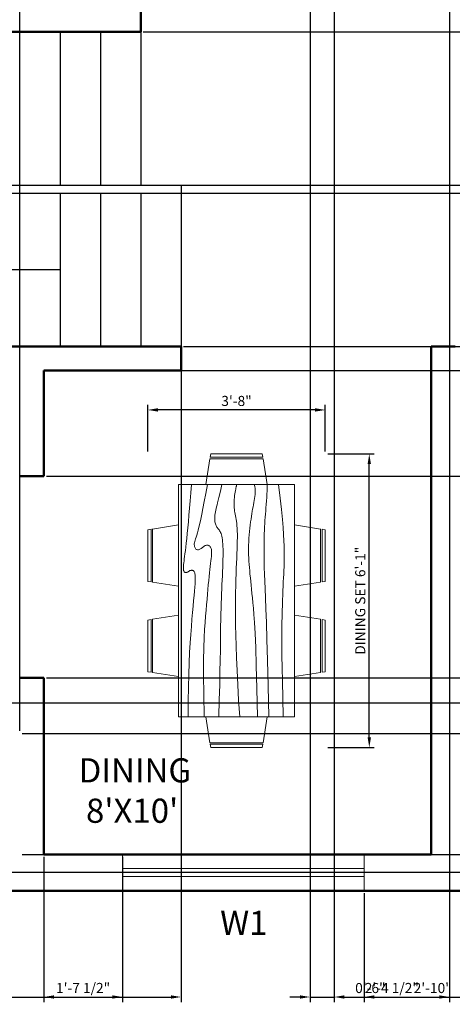
# Model space of a CAD drawing. Units: inches. Extents: x 2936 to 3364, y 2324 to 2867.
# Tile 2 of 4: x 3081 to 3188, y 2324 to 2568. Entities that reach past the tile are written whole.
import ezdxf

# ---------------------------------------------------------------- set-up
doc = ezdxf.new("R2010")
doc.units = ezdxf.units.IN
for name, color, linetype, lineweight in [('A-ANNO-DIMS', 2, 'Continuous', 18), ('A-ANNO-TEXT', 7, 'Continuous', 18), ('A-AREA-IDEN', 7, 'Continuous', 25), ('A-FLOR-STRS', 7, 'Continuous', 25), ('A-FURN', 8, 'Continuous', 18), ('A-GLAZ', 4, 'Continuous', 18), ('A-WALL', 7, 'Continuous', 50)]:
    doc.layers.add(name, color=color, linetype=linetype, lineweight=lineweight)
doc.styles.get("Standard").update_dxf_attribs({"font": 'arial.ttf'})
doc.dimstyles.new('ISO-25', dxfattribs={"dimtxt": 2.5, "dimasz": 2.5, "dimexe": 1.25, "dimexo": 0.625, "dimtad": 1, "dimdec": 0, "dimlunit": 4, "dimtxsty": 'Standard', "dimcen": 2.5, "dimadec": 0, "dimazin": 0, "dimtfac": 1, "dimtdec": 0, "dimtmove": 0, "dimatfit": 3, "dimfxl": 1, "dimarcsym": 0})

# ---------------------------------------------------------------- blocks, each defined once
blk = doc.blocks.new('Dining Set - 36 x 72 in.')
for p, q in [((-22, 27.5), (-22.1562, 26.50042)), ((-22, 27.5), (-6, 27.5)), ((-5.8437, 26.49966), (-6, 27.5)), ((6, 27.5), (5.8438, 26.50042)), ((6, 27.5), (22, 27.5)), ((22.1563, 26.49966), (22, 27.5)), ((-22.2343, 26.00059), (-23.4847, 17.99762)), ((-22.2304, 26), (-5.7608, 26)), ((-5.8416, 26.5), (-22.1534, 26.5)), ((-4.5152, 17.99762), (-5.7655, 25.99926)), ((5.7657, 26.00059), (4.5153, 17.99762)), ((5.7696, 26), (22.2392, 26)), ((22.1584, 26.5), (5.8466, 26.5)), ((23.4848, 17.99762), (22.2345, 25.99926)), ((36, 18), (-36, 18)), ((-36, 18), (-36, -18)), ((36, -18), (36, 18)), ((-44.0006, 8.23428), (-35.9976, 9.48474)), ((44.0006, 8.23428), (35.9976, 9.48474)), ((-45.5, 8), (-44.5004, 8.15617)), ((-45.5, 8), (-45.5, -8)), ((-44.5, -8.15843), (-44.5, 8.15338)), ((-44, 8.23041), (-44, -8.23915)), ((44, 8.23041), (44, -8.23915)), ((44.5, -8.15843), (44.5, 8.15338)), ((45.5, 8), (44.5005, 8.15617)), ((45.5, 8), (45.5, -8)), ((-44.4997, -8.15631), (-45.5, -8)), ((-35.9976, -9.48476), (-43.9993, -8.2345)), ((35.9976, -9.48476), (43.9993, -8.2345)), ((44.4997, -8.15631), (45.5, -8)), ((-36, -18), (36, -18)), ((-22.2343, -26.0006), (-23.4847, -17.99762)), ((-4.5152, -17.99762), (-5.7655, -25.99928)), ((5.7657, -26.0006), (4.5153, -17.99762)), ((23.4848, -17.99762), (22.2345, -25.99928)), ((-22.2304, -26), (-5.7608, -26)), ((-22, -27.5), (-22.1562, -26.50044)), ((-5.8416, -26.5), (-22.1534, -26.5)), ((-5.8437, -26.49967), (-6, -27.5)), ((5.7696, -26), (22.2392, -26)), ((6, -27.5), (5.8438, -26.50044)), ((22.1584, -26.5), (5.8466, -26.5)), ((22.1563, -26.49967), (22, -27.5)), ((-22, -27.5), (-6, -27.5)), ((6, -27.5), (22, -27.5))]:
    blk.add_line(p, q)
for points in [[(-36, 15), (-31.1772, 14.97754), (-26.8079, 14.91406), (-22.8538, 14.81543), (-19.276, 14.6875), (-16.0362, 14.53613), (-13.0957, 14.36718), (-10.4159, 14.18652), (-7.9583, 14), (-5.6904, 13.81315), (-3.6035, 13.63021), (-1.6954, 13.45508), (0.0365, 13.29166), (1.5945, 13.14388), (2.9811, 13.01562), (4.1988, 12.9108), (5.25, 12.83333), (6.1393, 12.78613), (6.8802, 12.76823), (7.4883, 12.77767), (7.9792, 12.8125), (8.3685, 12.87077), (8.6719, 12.95052), (8.9049, 13.0498), (9.0833, 13.16666), (9.2205, 13.29899), (9.3216, 13.44401), (9.3895, 13.59879), (9.4271, 13.76041), (9.4373, 13.92594), (9.4232, 14.09245), (9.3875, 14.257), (9.3333, 14.41666), (9.2638, 14.56917), (9.1836, 14.71484), (9.0975, 14.85465), (9.0104, 14.98958), (8.9272, 15.1206), (8.8529, 15.2487), (8.7922, 15.37483), (8.75, 15.5), (8.7305, 15.62467), (8.7344, 15.74739), (8.7617, 15.86621), (8.8125, 15.97916), (8.8867, 16.08431), (8.9844, 16.17968), (9.1055, 16.26334), (9.25, 16.33333), (9.4189, 16.38802), (9.6172, 16.42708), (9.8506, 16.45052), (10.125, 16.45833), (10.4463, 16.45052), (10.8203, 16.42708), (11.2529, 16.38802), (11.75, 16.33333), (12.3184, 16.26318), (12.9694, 16.17838), (13.7151, 16.07991), (14.5677, 15.96875), (15.5395, 15.84586), (16.6426, 15.71224), (17.8893, 15.56884), (19.2917, 15.41666), (20.859, 15.25667), (22.5879, 15.08984), (24.4721, 14.91715), (26.5052, 14.73958), (28.6809, 14.5581), (30.9929, 14.3737), (33.4347, 14.18733), (36, 14)], [(-36, 10), (-28.9766, 10.14274), (-23.1725, 10.20442), (-18.4241, 10.19775), (-14.5677, 10.13541), (-11.4399, 10.03011), (-8.877, 9.89453), (-6.7154, 9.74137), (-4.7917, 9.58333), (-2.9698, 9.43082), (-1.2246, 9.28515), (0.4415, 9.14534), (2.026, 9.01041), (3.5266, 8.87939), (4.9408, 8.7513), (6.266, 8.62516), (7.5, 8.5), (8.6411, 8.37549), (9.6914, 8.2539), (10.6538, 8.13818), (11.5312, 8.03125), (12.3267, 7.93603), (13.043, 7.85547), (13.6831, 7.79248), (14.25, 7.75), (14.7471, 7.7303), (15.1797, 7.73307), (15.5537, 7.75732), (15.875, 7.80208), (16.1494, 7.86637), (16.3828, 7.94922), (16.5811, 8.04964), (16.75, 8.16666), (16.8944, 8.29915), (17.0143, 8.44531), (17.1089, 8.60319), (17.1771, 8.77083), (17.218, 8.94629), (17.2305, 9.1276), (17.2137, 9.31282), (17.1667, 9.5), (17.0895, 9.6875), (16.987, 9.875), (16.8649, 10.0625), (16.7292, 10.25), (16.5856, 10.4375), (16.4401, 10.625), (16.2985, 10.8125), (16.1667, 11), (16.05, 11.18733), (15.9518, 11.3737), (15.8752, 11.5581), (15.8229, 11.73958), (15.798, 11.91715), (15.8034, 12.08984), (15.842, 12.25667), (15.9167, 12.41666), (16.0295, 12.56836), (16.1784, 12.70833), (16.3605, 12.83268), (16.5729, 12.9375), (16.8127, 13.01888), (17.0768, 13.07291), (17.3625, 13.0957), (17.6667, 13.08333), (17.9894, 13.03312), (18.3418, 12.94726), (18.7382, 12.82918), (19.1927, 12.68229), (19.7195, 12.51001), (20.3327, 12.31575), (21.0465, 12.10294), (21.875, 11.875), (22.8357, 11.63354), (23.959, 11.37304), (25.2786, 11.08618), (26.8282, 10.76562), (28.6414, 10.40405), (30.752, 9.99414), (33.1936, 9.52856), (36, 9)], [(-36, 5.5), (-30.7157, 5.3348), (-26.069, 5.20963), (-21.9946, 5.11767), (-18.4271, 5.05208), (-15.3009, 5.00602), (-12.5508, 4.97265), (-10.1112, 4.94515), (-7.9167, 4.91666), (-5.909, 4.88167), (-4.0586, 4.83984), (-2.3429, 4.79215), (-0.7396, 4.73958), (0.7739, 4.6831), (2.22, 4.6237), (3.6213, 4.56233), (5, 4.5), (6.373, 4.43782), (7.7344, 4.3776), (9.0723, 4.32129), (10.375, 4.27083), (11.6309, 4.22819), (12.8281, 4.19531), (13.9551, 4.17415), (15, 4.16666), (15.954, 4.17448), (16.819, 4.19791), (17.6001, 4.23698), (18.3021, 4.29166), (18.9299, 4.36198), (19.4883, 4.44791), (19.9823, 4.54948), (20.4167, 4.66666), (20.7969, 4.79899), (21.1302, 4.94401), (21.4245, 5.09879), (21.6875, 5.26041), (21.9271, 5.42594), (22.1511, 5.59245), (22.3672, 5.757), (22.5834, 5.91666), (22.8065, 6.06868), (23.0404, 6.21093), (23.2879, 6.34147), (23.5521, 6.45833), (23.8358, 6.55957), (24.142, 6.64323), (24.4735, 6.70735), (24.8334, 6.75), (25.2235, 6.76969), (25.642, 6.76692), (26.0858, 6.74267), (26.5521, 6.69791), (27.0379, 6.63362), (27.5404, 6.55078), (28.0565, 6.45036), (28.5834, 6.33333), (29.1242, 6.19987), (29.7071, 6.04687), (30.3661, 5.87044), (31.1354, 5.66666), (32.0493, 5.43164), (33.142, 5.16146), (34.4475, 4.85221), (36, 4.5)], [(-36, -1), (-30.7915, -0.6591), (-26.0195, -0.38216), (-21.6519, -0.16284), (-17.6563, 0.00521), (-14.0005, 0.12833), (-10.6523, 0.21289), (-7.5796, 0.26522), (-4.75, 0.29166), (-2.134, 0.29793), (0.2878, 0.28711), (2.5317, 0.26163), (4.6146, 0.22396), (6.5529, 0.17651), (8.3633, 0.12174), (10.0623, 0.06209), (11.6667, 0), (13.1899, -0.06201), (14.6341, -0.1211), (15.9982, -0.17432), (17.2813, -0.21875), (18.4823, -0.25147), (19.6003, -0.26953), (20.6343, -0.27002), (21.5834, -0.25), (22.4481, -0.20768), (23.2357, -0.14584), (23.9549, -0.06836), (24.6146, 0.02083), (25.2235, 0.11784), (25.7904, 0.21875), (26.3241, 0.31966), (26.8334, 0.41666), (27.3265, 0.50618), (27.8099, 0.58593), (28.2894, 0.65397), (28.7709, 0.70833), (29.2601, 0.74707), (29.763, 0.76823), (30.2855, 0.76985), (30.8334, 0.75), (31.4088, 0.70784), (31.9994, 0.64713), (32.589, 0.57275), (33.1615, 0.48958), (33.7008, 0.4025), (34.1908, 0.3164), (34.6153, 0.23616), (34.9584, 0.16666), (35.2099, 0.11165), (35.3848, 0.07031), (35.504, 0.04069), (35.5886, 0.02083), (35.6594, 0.00879), (35.7377, 0.0026), (35.8442, 0.00032), (36, 0)], [(-36, -6.5), (-27.1843, -6.31267), (-20.084, -6.1263), (-14.469, -5.9419), (-10.1094, -5.76042), (-6.7752, -5.58285), (-4.2363, -5.41016), (-2.2629, -5.24333), (-0.625, -5.08334), (0.8708, -4.93099), (2.2715, -4.78646), (3.5872, -4.64974), (4.8281, -4.52084), (6.0046, -4.39974), (7.127, -4.28646), (8.2053, -4.18099), (9.25, -4.08334), (10.2705, -3.99382), (11.2734, -3.91407), (12.2647, -3.84603), (13.25, -3.79167), (14.2354, -3.75293), (15.2266, -3.73177), (16.2295, -3.73015), (17.25, -3.75), (18.2912, -3.79248), (19.3451, -3.85547), (20.4009, -3.93604), (21.4479, -4.03125), (22.4754, -4.13819), (23.4727, -4.25391), (24.4289, -4.37549), (25.3334, -4.5), (26.1785, -4.62492), (26.9694, -4.74935), (27.7145, -4.87281), (28.4219, -4.99479), (29.1, -5.11483), (29.7572, -5.23242), (30.4016, -5.34709), (31.0417, -5.45834), (31.6837, -5.56437), (32.3262, -5.65821), (32.9658, -5.73153), (33.599, -5.77604), (34.2224, -5.78345), (34.8327, -5.74545), (35.4264, -5.65373), (36, -5.5)], [(-36, -10), (-26.4022, -9.81299), (-18.4675, -9.62891), (-11.9839, -9.45069), (-6.7396, -9.28125), (-2.5226, -9.12354), (0.8789, -8.98047), (3.6769, -8.85498), (6.0833, -8.75), (8.2767, -8.66765), (10.3021, -8.60677), (12.1712, -8.56543), (13.8958, -8.54167), (15.4876, -8.53353), (16.9583, -8.53907), (18.3197, -8.55632), (19.5834, -8.58334), (20.7616, -8.61841), (21.8685, -8.66081), (22.9188, -8.71004), (23.9271, -8.76563), (24.9081, -8.82707), (25.8763, -8.89388), (26.8465, -8.96558), (27.8334, -9.04167), (28.8474, -9.12118), (29.8828, -9.20117), (30.93, -9.27824), (31.9792, -9.34896), (33.0205, -9.40991), (34.0443, -9.45768), (35.0407, -9.48885), (36, -9.5)], [(-36, -14.5), (-30.0881, -14.33513), (-25.0332, -14.21224), (-20.7312, -14.12647), (-17.0781, -14.07292), (-13.97, -14.04671), (-11.3027, -14.04297), (-8.9724, -14.05681), (-6.875, -14.08334), (-4.9224, -14.11833), (-3.0905, -14.16016), (-1.3709, -14.20785), (0.2448, -14.26042), (1.7647, -14.3169), (3.1973, -14.3763), (4.5507, -14.43767), (5.8333, -14.5), (7.0554, -14.5621), (8.235, -14.62175), (9.3922, -14.67652), (10.5469, -14.72396), (11.7192, -14.76164), (12.929, -14.78711), (14.1965, -14.79794), (15.5417, -14.79167), (16.9933, -14.76424), (18.6152, -14.70508), (20.4804, -14.60197), (22.6615, -14.44271), (25.2312, -14.21509), (28.2624, -13.9069), (31.8277, -13.50594), (36, -13)]]:
    blk.add_lwpolyline(points)
blk = doc.blocks.new('WIN-W1-60IN')
for p, q in [((3.5, 60), (3.5, 0)), ((5.5, 60), (5.5, 0))]:
    blk.add_line(p, q)
blk.add_lwpolyline([(0, 0), (9, 0), (9, 60), (0, 60)], close=True)
blk = doc.blocks.new('*D27')
at = {"layer": 'A-ANNO-DIMS', "color": 0, "lineweight": -2, "transparency": 16777216}
for p, q in [((3157.56, 2460.42), (3169.1, 2460.42)), ((3167.85, 2390.13), (3167.85, 2457.92)), ((3157.56, 2387.63), (3169.1, 2387.63))]:
    blk.add_line(p, q, dxfattribs=at)
at = {"layer": 'A-ANNO-DIMS', "color": 0, "transparency": 16777216}
for points in [[(3167.44, 2457.92), (3168.27, 2457.92), (3167.85, 2460.42)], [(3167.44, 2390.13), (3168.27, 2390.13), (3167.85, 2387.63)]]:
    blk.add_solid(points, dxfattribs=at)
at = {"layer": 'Defpoints', "color": 0, "transparency": 16777216}
for p in [(3156.93, 2460.42), (3167.85, 2460.42), (3156.93, 2387.63)]:
    blk.add_point(p, dxfattribs=at)
at = {"layer": 'A-ANNO-DIMS', "color": 0, "transparency": 16777216, "insert": (3165.94, 2424.03), "char_height": 2.5, "attachment_point": 5, "rotation": 90}
blk.add_mtext('DINING SET 6\'-1"', dxfattribs=at)
blk = doc.blocks.new('*D28')
at = {"layer": 'A-ANNO-DIMS', "color": 0, "lineweight": -2, "transparency": 16777216}
for p, q in [((3112.94, 2461.05), (3112.94, 2472.59)), ((3154.43, 2471.34), (3115.44, 2471.34)), ((3156.93, 2461.05), (3156.93, 2472.59))]:
    blk.add_line(p, q, dxfattribs=at)
at = {"layer": 'A-ANNO-DIMS', "color": 0, "transparency": 16777216}
for points in [[(3115.44, 2471.76), (3115.44, 2470.93), (3112.94, 2471.34)], [(3154.43, 2471.76), (3154.43, 2470.93), (3156.93, 2471.34)]]:
    blk.add_solid(points, dxfattribs=at)
at = {"layer": 'Defpoints', "color": 0, "transparency": 16777216}
for p in [(3112.94, 2471.34), (3112.94, 2460.42), (3156.93, 2460.42)]:
    blk.add_point(p, dxfattribs=at)
at = {"layer": 'A-ANNO-DIMS', "color": 0, "transparency": 16777216, "insert": (3134.93, 2473.25), "char_height": 2.5, "attachment_point": 5}
blk.add_mtext('3\'-8"', dxfattribs=at)
blk = doc.blocks.new('*D45')
at = {"layer": 'A-ANNO-DIMS', "color": 0, "lineweight": -2, "transparency": 16777216}
for p, q in [((3087.17, 2360.49), (3087.17, 2324.51)), ((3106.62, 2360.49), (3106.62, 2324.51)), ((3089.67, 2325.76), (3104.12, 2325.76))]:
    blk.add_line(p, q, dxfattribs=at)
at = {"layer": 'A-ANNO-DIMS', "color": 0, "transparency": 16777216}
for points in [[(3089.67, 2326.18), (3089.67, 2325.35), (3087.17, 2325.76)], [(3104.12, 2326.18), (3104.12, 2325.35), (3106.62, 2325.76)]]:
    blk.add_solid(points, dxfattribs=at)
at = {"layer": 'Defpoints', "color": 0, "transparency": 16777216}
for p in [(3087.17, 2361.11), (3106.62, 2361.11), (3106.62, 2325.76)]:
    blk.add_point(p, dxfattribs=at)
at = {"layer": 'A-ANNO-DIMS', "color": 0, "transparency": 16777216, "insert": (3096.89, 2327.68), "char_height": 2.5, "attachment_point": 5}
blk.add_mtext('1\'-7 1/2"', dxfattribs=at)
blk = doc.blocks.new('*D46')
at = {"layer": 'A-ANNO-DIMS', "color": 0, "lineweight": -2, "transparency": 16777216}
for p, q in [((3166.62, 2351.49), (3166.62, 2324.51)), ((3200.55, 2351.49), (3200.55, 2324.51)), ((3169.12, 2325.76), (3198.05, 2325.76))]:
    blk.add_line(p, q, dxfattribs=at)
at = {"layer": 'A-ANNO-DIMS', "color": 0, "transparency": 16777216}
for points in [[(3169.12, 2326.18), (3169.12, 2325.35), (3166.62, 2325.76)], [(3198.05, 2326.18), (3198.05, 2325.35), (3200.55, 2325.76)]]:
    blk.add_solid(points, dxfattribs=at)
at = {"layer": 'Defpoints', "color": 0, "transparency": 16777216}
for p in [(3166.62, 2352.11), (3200.55, 2352.11), (3200.55, 2325.76)]:
    blk.add_point(p, dxfattribs=at)
at = {"layer": 'A-ANNO-DIMS', "color": 0, "transparency": 16777216, "insert": (3183.58, 2327.67), "char_height": 2.5, "attachment_point": 5}
blk.add_mtext('2\'-10"', dxfattribs=at)
blk = doc.blocks.new('*D50')
at = {"layer": 'A-ANNO-DIMS', "color": 0, "lineweight": -2, "transparency": 16777216}
for p, q in [((3121.79, 2525.11), (3363.77, 2525.11)), ((3362.52, 2489.61), (3362.52, 2522.61)), ((3121.79, 2487.11), (3363.77, 2487.11))]:
    blk.add_line(p, q, dxfattribs=at)
at = {"layer": 'A-ANNO-DIMS', "color": 0, "transparency": 16777216}
for points in [[(3362.1, 2522.61), (3362.94, 2522.61), (3362.52, 2525.11)], [(3362.1, 2489.61), (3362.94, 2489.61), (3362.52, 2487.11)]]:
    blk.add_solid(points, dxfattribs=at)
at = {"layer": 'Defpoints', "color": 0, "transparency": 16777216}
for p in [(3121.17, 2525.11), (3362.52, 2525.11), (3121.17, 2487.11)]:
    blk.add_point(p, dxfattribs=at)
at = {"layer": 'A-ANNO-DIMS', "color": 0, "transparency": 16777216, "insert": (3360.62, 2506.11), "char_height": 2.5, "attachment_point": 5, "rotation": 90}
blk.add_mtext('3\'-2"', dxfattribs=at)
blk = doc.blocks.new('*D51')
at = {"layer": 'A-ANNO-DIMS', "color": 0, "lineweight": -2, "transparency": 16777216}
for p, q in [((3153.17, 2822.49), (3153.17, 2324.51)), ((3159.17, 2822.49), (3159.17, 2324.51)), ((3150.67, 2325.76), (3148.17, 2325.76)), ((3153.17, 2325.76), (3159.17, 2325.76)), ((3161.67, 2325.76), (3172.07, 2325.76))]:
    blk.add_line(p, q, dxfattribs=at)
at = {"layer": 'A-ANNO-DIMS', "color": 0, "transparency": 16777216}
for points in [[(3150.67, 2326.18), (3150.67, 2325.35), (3153.17, 2325.76)], [(3161.67, 2326.18), (3161.67, 2325.35), (3159.17, 2325.76)]]:
    blk.add_solid(points, dxfattribs=at)
at = {"layer": 'Defpoints', "color": 0, "transparency": 16777216}
for p in [(3153.17, 2823.11), (3159.17, 2823.11), (3159.17, 2325.76)]:
    blk.add_point(p, dxfattribs=at)
at = {"layer": 'A-ANNO-DIMS', "color": 0, "transparency": 16777216, "insert": (3168.12, 2327.67), "char_height": 2.5, "attachment_point": 5}
blk.add_mtext('0\'-6"', dxfattribs=at)
blk = doc.blocks.new('*D53')
at = {"layer": 'A-ANNO-DIMS', "color": 0, "lineweight": -2, "transparency": 16777216}
for p, q in [((3159.17, 2739.18), (3159.17, 2324.51)), ((3187.71, 2739.18), (3187.71, 2324.51)), ((3161.67, 2325.76), (3185.21, 2325.76))]:
    blk.add_line(p, q, dxfattribs=at)
at = {"layer": 'A-ANNO-DIMS', "color": 0, "transparency": 16777216}
for points in [[(3161.67, 2326.18), (3161.67, 2325.35), (3159.17, 2325.76)], [(3185.21, 2326.18), (3185.21, 2325.35), (3187.71, 2325.76)]]:
    blk.add_solid(points, dxfattribs=at)
at = {"layer": 'Defpoints', "color": 0, "transparency": 16777216}
for p in [(3159.17, 2739.81), (3187.71, 2739.81), (3187.71, 2325.76)]:
    blk.add_point(p, dxfattribs=at)
at = {"layer": 'A-ANNO-DIMS', "color": 0, "transparency": 16777216, "insert": (3173.44, 2327.68), "char_height": 2.5, "attachment_point": 5}
blk.add_mtext('2\'-4 1/2"', dxfattribs=at)
blk = doc.blocks.new('*D54')
at = {"layer": 'A-ANNO-DIMS', "color": 0, "lineweight": -2, "transparency": 16777216}
for p, q in [((3087.79, 2454.95), (3363.77, 2454.95)), ((3362.52, 2407.37), (3362.52, 2452.45)), ((3087.79, 2404.87), (3363.77, 2404.87))]:
    blk.add_line(p, q, dxfattribs=at)
at = {"layer": 'A-ANNO-DIMS', "color": 0, "transparency": 16777216}
for points in [[(3362.1, 2452.45), (3362.94, 2452.45), (3362.52, 2454.95)], [(3362.1, 2407.37), (3362.94, 2407.37), (3362.52, 2404.87)]]:
    blk.add_solid(points, dxfattribs=at)
at = {"layer": 'Defpoints', "color": 0, "transparency": 16777216}
for p in [(3087.17, 2454.95), (3362.52, 2454.95), (3087.17, 2404.87)]:
    blk.add_point(p, dxfattribs=at)
at = {"layer": 'A-ANNO-DIMS', "color": 0, "transparency": 16777216, "insert": (3360.64, 2429.91), "char_height": 2.5, "attachment_point": 5, "rotation": 90}
blk.add_mtext('4\'-2"', dxfattribs=at)
blk = doc.blocks.new('*D55')
at = {"layer": 'A-ANNO-DIMS', "color": 0, "lineweight": -2, "transparency": 16777216}
for p, q in [((3087.79, 2481.11), (3363.77, 2481.11)), ((3362.52, 2457.45), (3362.52, 2478.61)), ((3087.79, 2454.95), (3363.77, 2454.95))]:
    blk.add_line(p, q, dxfattribs=at)
at = {"layer": 'A-ANNO-DIMS', "color": 0, "transparency": 16777216}
for points in [[(3362.1, 2478.61), (3362.94, 2478.61), (3362.52, 2481.11)], [(3362.1, 2457.45), (3362.94, 2457.45), (3362.52, 2454.95)]]:
    blk.add_solid(points, dxfattribs=at)
at = {"layer": 'Defpoints', "color": 0, "transparency": 16777216}
for p in [(3087.17, 2481.11), (3362.52, 2481.11), (3087.17, 2454.95)]:
    blk.add_point(p, dxfattribs=at)
at = {"layer": 'A-ANNO-DIMS', "color": 0, "transparency": 16777216, "insert": (3360.64, 2468.03), "char_height": 2.5, "attachment_point": 5, "rotation": 90}
blk.add_mtext('2\'-2"', dxfattribs=at)
blk = doc.blocks.new('*D56')
at = {"layer": 'A-ANNO-DIMS', "color": 0, "lineweight": -2, "transparency": 16777216}
for p, q in [((3081.79, 2391.11), (3363.77, 2391.11)), ((3362.52, 2388.61), (3362.52, 2363.61)), ((3081.79, 2361.11), (3363.77, 2361.11))]:
    blk.add_line(p, q, dxfattribs=at)
at = {"layer": 'A-ANNO-DIMS', "color": 0, "transparency": 16777216}
for points in [[(3362.1, 2388.61), (3362.94, 2388.61), (3362.52, 2391.11)], [(3362.1, 2363.61), (3362.94, 2363.61), (3362.52, 2361.11)]]:
    blk.add_solid(points, dxfattribs=at)
at = {"layer": 'Defpoints', "color": 0, "transparency": 16777216}
for p in [(3081.17, 2391.11), (3081.17, 2361.11), (3362.52, 2361.11)]:
    blk.add_point(p, dxfattribs=at)
at = {"layer": 'A-ANNO-DIMS', "color": 0, "transparency": 16777216, "insert": (3360.62, 2376.11), "char_height": 2.5, "attachment_point": 5, "rotation": 90}
blk.add_mtext('2\'-6"', dxfattribs=at)
blk = doc.blocks.new('*D58')
at = {"layer": 'A-ANNO-DIMS', "color": 0, "lineweight": -2, "transparency": 16777216}
for p, q in [((3021.17, 2486.49), (3021.17, 2324.51)), ((3121.17, 2486.49), (3121.17, 2324.51)), ((3023.67, 2325.76), (3118.67, 2325.76))]:
    blk.add_line(p, q, dxfattribs=at)
at = {"layer": 'A-ANNO-DIMS', "color": 0, "transparency": 16777216}
for points in [[(3023.67, 2326.18), (3023.67, 2325.35), (3021.17, 2325.76)], [(3118.67, 2326.18), (3118.67, 2325.35), (3121.17, 2325.76)]]:
    blk.add_solid(points, dxfattribs=at)
at = {"layer": 'Defpoints', "color": 0, "transparency": 16777216}
for p in [(3021.17, 2487.11), (3121.17, 2487.11), (3121.17, 2325.76)]:
    blk.add_point(p, dxfattribs=at)
at = {"layer": 'A-ANNO-DIMS', "color": 0, "transparency": 16777216, "insert": (3071.17, 2327.67), "char_height": 2.5, "attachment_point": 5}
blk.add_mtext('8\'-4"', dxfattribs=at)
blk = doc.blocks.new('*D59')
at = {"layer": 'A-ANNO-DIMS', "color": 0, "lineweight": -2, "transparency": 16777216}
for p, q in [((3111.79, 2565.11), (3363.77, 2565.11)), ((3362.52, 2529.61), (3362.52, 2562.61)), ((3111.79, 2527.11), (3363.77, 2527.11))]:
    blk.add_line(p, q, dxfattribs=at)
at = {"layer": 'A-ANNO-DIMS', "color": 0, "transparency": 16777216}
for points in [[(3362.1, 2562.61), (3362.94, 2562.61), (3362.52, 2565.11)], [(3362.1, 2529.61), (3362.94, 2529.61), (3362.52, 2527.11)]]:
    blk.add_solid(points, dxfattribs=at)
at = {"layer": 'Defpoints', "color": 0, "transparency": 16777216}
for p in [(3111.17, 2565.11), (3362.52, 2565.11), (3111.17, 2527.11)]:
    blk.add_point(p, dxfattribs=at)
at = {"layer": 'A-ANNO-DIMS', "color": 0, "transparency": 16777216, "insert": (3360.62, 2546.11), "char_height": 2.5, "attachment_point": 5, "rotation": 90}
blk.add_mtext('3\'-2"', dxfattribs=at)
blk = doc.blocks.new('*D60')
at = {"layer": 'A-ANNO-DIMS', "color": 0, "lineweight": -2, "transparency": 16777216}
for p, q in [((3362.52, 2529.61), (3362.52, 2540.01)), ((3111.79, 2527.11), (3363.77, 2527.11)), ((3362.52, 2525.11), (3362.52, 2527.11)), ((3111.79, 2525.11), (3363.77, 2525.11)), ((3362.52, 2522.61), (3362.52, 2520.11))]:
    blk.add_line(p, q, dxfattribs=at)
at = {"layer": 'A-ANNO-DIMS', "color": 0, "transparency": 16777216}
for points in [[(3362.1, 2529.61), (3362.94, 2529.61), (3362.52, 2527.11)], [(3362.1, 2522.61), (3362.94, 2522.61), (3362.52, 2525.11)]]:
    blk.add_solid(points, dxfattribs=at)
at = {"layer": 'Defpoints', "color": 0, "transparency": 16777216}
for p in [(3111.17, 2527.11), (3362.52, 2527.11), (3111.17, 2525.11)]:
    blk.add_point(p, dxfattribs=at)
at = {"layer": 'A-ANNO-DIMS', "color": 0, "transparency": 16777216, "insert": (3360.62, 2536.06), "char_height": 2.5, "attachment_point": 5, "rotation": 90}
blk.add_mtext('0\'-2"', dxfattribs=at)
blk = doc.blocks.new('*D62')
at = {"layer": 'A-ANNO-DIMS', "color": 0, "lineweight": -2, "transparency": 16777216}
for p, q in [((3072.03, 2387.74), (3072.03, 2859.71)), ((3081.17, 2391.74), (3081.17, 2859.71)), ((3078.67, 2858.46), (3074.53, 2858.46))]:
    blk.add_line(p, q, dxfattribs=at)
at = {"layer": 'A-ANNO-DIMS', "color": 0, "transparency": 16777216}
for points in [[(3074.53, 2858.88), (3074.53, 2858.05), (3072.03, 2858.46)], [(3078.67, 2858.88), (3078.67, 2858.05), (3081.17, 2858.46)]]:
    blk.add_solid(points, dxfattribs=at)
at = {"layer": 'Defpoints', "color": 0, "transparency": 16777216}
for p in [(3072.03, 2858.46), (3081.17, 2391.11), (3072.03, 2387.11)]:
    blk.add_point(p, dxfattribs=at)
at = {"layer": 'A-ANNO-DIMS', "color": 0, "transparency": 16777216, "insert": (3076.6, 2860.37), "char_height": 2.5, "attachment_point": 5}
blk.add_mtext('0\'-9"', dxfattribs=at)
blk = doc.blocks.new('*D64')
at = {"layer": 'A-ANNO-DIMS', "color": 0, "lineweight": -2, "transparency": 16777216}
for p, q in [((3324.54, 2398.61), (2948.57, 2398.61)), ((2949.82, 2359.11), (2949.82, 2396.11)), ((3324.54, 2356.61), (2948.57, 2356.61))]:
    blk.add_line(p, q, dxfattribs=at)
at = {"layer": 'A-ANNO-DIMS', "color": 0, "transparency": 16777216}
for points in [[(2949.4, 2396.11), (2950.24, 2396.11), (2949.82, 2398.61)], [(2949.4, 2359.11), (2950.24, 2359.11), (2949.82, 2356.61)]]:
    blk.add_solid(points, dxfattribs=at)
at = {"layer": 'Defpoints', "color": 0, "transparency": 16777216}
for p in [(2949.82, 2398.61), (3325.17, 2398.61), (3325.17, 2356.61)]:
    blk.add_point(p, dxfattribs=at)
at = {"layer": 'A-ANNO-DIMS', "color": 0, "transparency": 16777216, "insert": (2947.92, 2377.61), "char_height": 2.5, "attachment_point": 5, "rotation": 90}
blk.add_mtext('3\'-6"', dxfattribs=at)

msp = doc.modelspace()

# ---------------------------------------------------------------- linework, layer by layer
at = {"layer": 'A-FLOR-STRS'}
for p, q in [((3091.17, 2565.11), (3091.17, 2527.11)), ((3101.17, 2565.11), (3101.17, 2527.11)), ((3111.17, 2565.11), (3111.17, 2527.11)), ((3021.17, 2527.11), (3121.17, 2527.11)), ((3121.17, 2527.11), (3121.17, 2487.11)), ((3021.17, 2525.11), (3121.17, 2525.11)), ((3091.17, 2525.11), (3091.17, 2487.11)), ((3101.17, 2525.11), (3101.17, 2487.11)), ((3111.17, 2525.11), (3111.17, 2487.11)), ((3091.17, 2506.11), (3007.29, 2506.11))]:
    msp.add_line(p, q, dxfattribs=at)
at = {"layer": 'A-WALL'}
for p, q in [((3111.17, 2571.11), (3111.17, 2565.11)), ((3111.17, 2565.11), (2985.17, 2565.11)), ((2985.17, 2487.11), (3121.17, 2487.11)), ((3121.17, 2487.11), (3121.17, 2481.11)), ((3183.17, 2487.11), (3183.17, 2361.11)), ((3183.17, 2487.11), (3189.17, 2487.11)), ((3087.17, 2481.11), (3087.17, 2454.95)), ((3087.17, 2481.11), (3121.17, 2481.11)), ((3081.17, 2454.95), (3087.17, 2454.95)), ((3081.17, 2404.87), (3087.17, 2404.87)), ((3087.17, 2404.87), (3087.17, 2361.11)), ((3087.17, 2361.11), (3183.17, 2361.11))]:
    msp.add_line(p, q, dxfattribs=at)
msp.add_lwpolyline([(3336.17, 2352.11), (3336.17, 2832.11), (2976.17, 2832.11), (2976.17, 2352.11), (3279.17, 2352.11)], dxfattribs=at)

# ---------------------------------------------------------------- block references
at = {"layer": 'A-FURN', "xscale": 0.7999530851733067, "yscale": 0.7999530851733067, "zscale": 0.7999530851733067, "rotation": 90}
msp.add_blockref('Dining Set - 36 x 72 in.', (3134.93, 2424.03), dxfattribs=at)
at = {"layer": 'A-GLAZ', "rotation": 90.00000000000088}
msp.add_blockref('WIN-W1-60IN', (3166.62, 2352.11), dxfattribs=at)

# ---------------------------------------------------------------- texts
at = {"layer": 'A-ANNO-TEXT', "insert": (3130.88, 2347.16), "char_height": 6, "attachment_point": 1}
msp.add_mtext_dynamic_manual_height_columns('W1', width=56.3393, gutter_width=12.5, heights=[0], dxfattribs=at)
at = {"layer": 'A-AREA-IDEN', "insert": (3095.78, 2384.96), "char_height": 6, "attachment_point": 1}
msp.add_mtext_dynamic_manual_height_columns("DINING \\P 8'X10'", width=56.3393, gutter_width=12.5, heights=[0], dxfattribs=at)

# ---------------------------------------------------------------- dimensions: what is measured, and where the dimension line sits
at = {"layer": 'A-ANNO-DIMS'}
for base, p1, p2, picture, middle in [((3072.03, 2858.46), (3081.17, 2391.11), (3072.03, 2387.11), '*D62', (3076.6, 2860.37)), ((3159.17, 2325.76), (3153.17, 2823.11), (3159.17, 2823.11), '*D51', (3168.12, 2327.67)), ((3187.71, 2325.76), (3159.17, 2739.81), (3187.71, 2739.81), '*D53', (3173.44, 2327.68)), ((3121.17, 2325.76), (3021.17, 2487.11), (3121.17, 2487.11), '*D58', (3071.17, 2327.67)), ((3106.6162, 2325.764), (3087.1697, 2361.114), (3106.6162, 2361.114), '*D45', (3096.8929, 2327.6816)), ((3200.55, 2325.76), (3166.62, 2352.11), (3200.55, 2352.11), '*D46', (3183.58, 2327.67))]:
    dim = msp.add_linear_dim(base=base, p1=p1, p2=p2, dimstyle='ISO-25', override={"dimdec": 1, "dimlfac": 1, "dimrnd": 0, "dimzin": 1, "dimdsep": 46, "dimlunit": 4, "dimfrac": 2}, dxfattribs=at)
    dim.commit()
    dim.dimension.update_dxf_attribs({"geometry": picture, "text_midpoint": middle})
for base, p1, p2, angle, picture, middle in [((3362.52, 2565.11), (3111.17, 2527.11), (3111.17, 2565.11), 90, '*D59', (3360.62, 2546.11)), ((3362.52, 2527.11), (3111.17, 2525.11), (3111.17, 2527.11), 90, '*D60', (3360.62, 2536.06)), ((3362.52, 2525.11), (3121.17, 2487.11), (3121.17, 2525.11), 90, '*D50', (3360.62, 2506.11)), ((3362.52, 2481.11), (3087.17, 2454.95), (3087.17, 2481.11), 90, '*D55', (3360.64, 2468.03)), ((3112.94, 2471.34), (3156.93, 2460.42), (3112.94, 2460.42), 180, '*D28', (3134.93, 2473.25)), ((3362.52, 2454.95), (3087.17, 2404.87), (3087.17, 2454.95), 90, '*D54', (3360.64, 2429.91)), ((2949.82, 2398.61), (3325.17, 2356.61), (3325.17, 2398.61), 90, '*D64', (2947.92, 2377.61)), ((3362.52, 2361.11), (3081.17, 2391.11), (3081.17, 2361.11), 90, '*D56', (3360.62, 2376.11))]:
    dim = msp.add_linear_dim(base=base, p1=p1, p2=p2, angle=angle, dimstyle='ISO-25', override={"dimdec": 1, "dimlfac": 1, "dimrnd": 0, "dimzin": 1, "dimdsep": 46, "dimlunit": 4, "dimfrac": 2}, dxfattribs=at)
    dim.commit()
    dim.dimension.update_dxf_attribs({"geometry": picture, "text_midpoint": middle})
dim = msp.add_linear_dim(base=(3167.85, 2460.42), p1=(3156.93, 2387.63), p2=(3156.93, 2460.42), angle=90, text='DINING SET <>', dimstyle='ISO-25', override={"dimdec": 1, "dimlfac": 1, "dimrnd": 0, "dimzin": 1, "dimdsep": 46, "dimlunit": 4, "dimfrac": 2}, dxfattribs=at)
dim.commit()
dim.dimension.update_dxf_attribs({"geometry": '*D27', "text_midpoint": (3165.94, 2424.03)})

doc.saveas('drawing.dxf')
